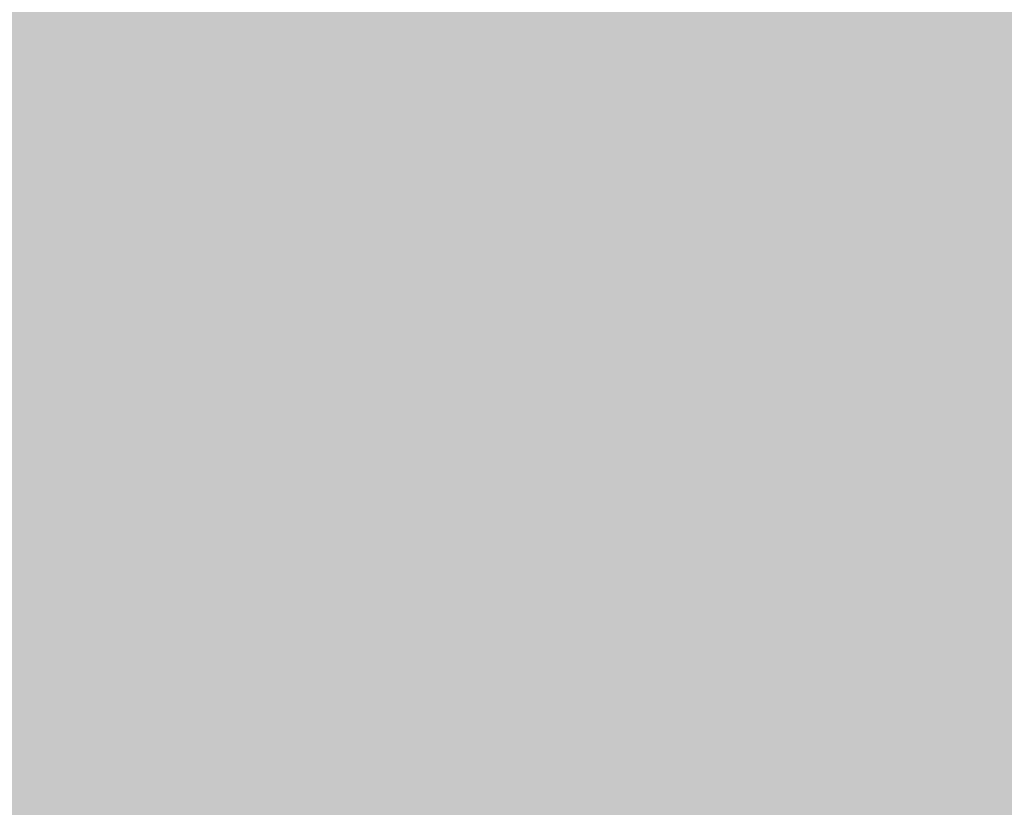
# Model space of a CAD drawing. Units: millimetres. Extents: x -22994 to 29398, y -19990 to 20176.
# Tile 102 of 135: x 229.428 to 231.767, y 85.199 to 87.071. Entities that reach past the tile are written whole.
import ezdxf
from ezdxf import colors
from ezdxf.entities.mleader import LeaderData, LeaderLine
from ezdxf.math import Vec2, Vec3

# ---------------------------------------------------------------- set-up
doc = ezdxf.new("R2010")
doc.units = ezdxf.units.MM
doc.header["$MEASUREMENT"] = 0
doc.layers.add('M-ANNO-TEXT', color=7, linetype='Continuous', lineweight=25)
doc.layers.add('M-DIMS', color=2, linetype='Continuous', lineweight=18)
doc.styles.get("Standard").update_dxf_attribs({"font": 'arial.ttf'})
doc.dimstyles.get("Standard").update_dxf_attribs({"dimtxt": 0.18, "dimasz": 10000, "dimexe": 0.18, "dimexo": 0.0625, "dimgap": 0.09, "dimtad": 0, "dimtih": 1, "dimtoh": 1, "dimdec": 0, "dimzin": 0, "dimdsep": 46, "dimtxsty": 'Standard', "dimcen": 0.09, "dimadec": 0, "dimazin": 0, "dimtfac": 1, "dimtdec": 0, "dimtofl": 0, "dimtmove": 0, "dimatfit": 3, "dimfxl": 1, "dimtolj": 1, "dimtzin": 0, "dimlwd": 30, "dimarcsym": 0})

# ---------------------------------------------------------------- blocks, each defined once
blk = doc.blocks.new('*D2')
at = {"layer": 'Defpoints', "color": 0, "transparency": 16777216}
for p in [(6.6773, 10.2713), (290.852, 10.2713), (290.852, -5.0787)]:
    blk.add_point(p, dxfattribs=at)
at = {"layer": 'M-DIMS', "color": 0, "lineweight": -2, "transparency": 16777216}
for p, q in [((6.6773, 10.2088), (6.6773, -5.2587)), ((290.852, 10.2088), (290.852, -5.2587))]:
    blk.add_line(p, q, dxfattribs=at)
at = {"layer": 'M-DIMS', "color": 0, "lineweight": 30, "transparency": 16777216}
for p, q in [((-9993.3227, -5.0787), (-19993.3227, -5.0787)), ((10290.852, -5.0787), (20290.852, -5.0787))]:
    blk.add_line(p, q, dxfattribs=at)
at = {"layer": 'M-DIMS', "color": 0, "transparency": 16777216}
for points in [[(-9993.3227, 1661.5879), (-9993.3227, -1671.7454), (6.6773, -5.0787)], [(10290.852, 1661.5879), (10290.852, -1671.7454), (290.852, -5.0787)]]:
    blk.add_solid(points, dxfattribs=at)
at = {"layer": 'M-DIMS', "color": 0, "transparency": 16777216, "insert": (148.7647, -5.0787), "char_height": 0.18, "attachment_point": 5}
blk.add_mtext('\\A1;284.2', dxfattribs=at)
blk = doc.blocks.new('*D3')
at = {"layer": 'Defpoints', "color": 0, "transparency": 16777216}
for p in [(110.2647, 204.1654), (110.2647, 176.3662), (95.8327, 127.967)]:
    blk.add_point(p, dxfattribs=at)
at = {"layer": 'M-DIMS', "color": 0, "lineweight": -2, "transparency": 16777216}
for p, q in [((95.8327, 128.0295), (95.8327, 204.3454)), ((110.2647, 176.4287), (110.2647, 204.3454))]:
    blk.add_line(p, q, dxfattribs=at)
at = {"layer": 'M-DIMS', "color": 0, "lineweight": 30, "transparency": 16777216}
for p, q in [((-9904.1673, 204.1654), (-19904.1673, 204.1654)), ((10110.2647, 204.1654), (20110.2647, 204.1654))]:
    blk.add_line(p, q, dxfattribs=at)
at = {"layer": 'M-DIMS', "color": 0, "transparency": 16777216}
for points in [[(-9904.1673, 1870.8321), (-9904.1673, -1462.5013), (95.8327, 204.1654)], [(10110.2647, 1870.8321), (10110.2647, -1462.5013), (110.2647, 204.1654)]]:
    blk.add_solid(points, dxfattribs=at)
at = {"layer": 'M-DIMS', "color": 0, "transparency": 16777216, "insert": (103.0487, 204.1654), "char_height": 0.18, "attachment_point": 5}
blk.add_mtext('\\A1;14.432', dxfattribs=at)
blk = doc.blocks.new('*D4')
at = {"layer": 'Defpoints', "color": 0, "transparency": 16777216}
for p in [(116.2647, 204.1654), (110.2647, 176.3662), (116.2647, 176.3662)]:
    blk.add_point(p, dxfattribs=at)
at = {"layer": 'M-DIMS', "color": 0, "lineweight": -2, "transparency": 16777216}
for p, q in [((110.2647, 176.4287), (110.2647, 204.3454)), ((116.2647, 176.4287), (116.2647, 204.3454))]:
    blk.add_line(p, q, dxfattribs=at)
at = {"layer": 'M-DIMS', "color": 0, "lineweight": 30, "transparency": 16777216}
for p, q in [((-9889.7353, 204.1654), (-19889.7353, 204.1654)), ((10116.2647, 204.1654), (20116.2647, 204.1654))]:
    blk.add_line(p, q, dxfattribs=at)
at = {"layer": 'M-DIMS', "color": 0, "transparency": 16777216}
for points in [[(-9889.7353, 1870.8321), (-9889.7353, -1462.5013), (110.2647, 204.1654)], [(10116.2647, 1870.8321), (10116.2647, -1462.5013), (116.2647, 204.1654)]]:
    blk.add_solid(points, dxfattribs=at)
at = {"layer": 'M-DIMS', "color": 0, "transparency": 16777216, "insert": (113.2647, 204.1654), "char_height": 0.18, "attachment_point": 5}
blk.add_mtext('\\A1;6', dxfattribs=at)
blk = doc.blocks.new('*D5')
at = {"layer": 'Defpoints', "color": 0, "transparency": 16777216}
for p in [(181.2647, 204.1654), (116.2647, 176.3662), (181.2647, 176.3662)]:
    blk.add_point(p, dxfattribs=at)
at = {"layer": 'M-DIMS', "color": 0, "lineweight": -2, "transparency": 16777216}
for p, q in [((116.2647, 176.4287), (116.2647, 204.3454)), ((181.2647, 176.4287), (181.2647, 204.3454))]:
    blk.add_line(p, q, dxfattribs=at)
at = {"layer": 'M-DIMS', "color": 0, "lineweight": 30, "transparency": 16777216}
for p, q in [((-9883.7353, 204.1654), (-19883.7353, 204.1654)), ((10181.2647, 204.1654), (20181.2647, 204.1654))]:
    blk.add_line(p, q, dxfattribs=at)
at = {"layer": 'M-DIMS', "color": 0, "transparency": 16777216}
for points in [[(-9883.7353, 1870.8321), (-9883.7353, -1462.5013), (116.2647, 204.1654)], [(10181.2647, 1870.8321), (10181.2647, -1462.5013), (181.2647, 204.1654)]]:
    blk.add_solid(points, dxfattribs=at)
at = {"layer": 'M-DIMS', "color": 0, "transparency": 16777216, "insert": (148.7647, 204.1654), "char_height": 0.18, "attachment_point": 5}
blk.add_mtext('\\A1;65', dxfattribs=at)
blk = doc.blocks.new('*D6')
at = {"layer": 'Defpoints', "color": 0, "transparency": 16777216}
for p in [(187.2647, 204.1654), (181.2647, 176.3662), (187.2647, 176.3662)]:
    blk.add_point(p, dxfattribs=at)
at = {"layer": 'M-DIMS', "color": 0, "lineweight": -2, "transparency": 16777216}
for p, q in [((181.2647, 176.4287), (181.2647, 204.3454)), ((187.2647, 176.4287), (187.2647, 204.3454))]:
    blk.add_line(p, q, dxfattribs=at)
at = {"layer": 'M-DIMS', "color": 0, "lineweight": 30, "transparency": 16777216}
for p, q in [((-9818.7353, 204.1654), (-19818.7353, 204.1654)), ((10187.2647, 204.1654), (20187.2647, 204.1654))]:
    blk.add_line(p, q, dxfattribs=at)
at = {"layer": 'M-DIMS', "color": 0, "transparency": 16777216}
for points in [[(-9818.7353, 1870.8321), (-9818.7353, -1462.5013), (181.2647, 204.1654)], [(10187.2647, 1870.8321), (10187.2647, -1462.5013), (187.2647, 204.1654)]]:
    blk.add_solid(points, dxfattribs=at)
at = {"layer": 'M-DIMS', "color": 0, "transparency": 16777216, "insert": (184.2647, 204.1654), "char_height": 0.18, "attachment_point": 5}
blk.add_mtext('\\A1;6', dxfattribs=at)
blk = doc.blocks.new('*D7')
at = {"layer": 'Defpoints', "color": 0, "transparency": 16777216}
for p in [(201.6967, 204.1654), (187.2647, 176.3662), (201.6967, 127.967)]:
    blk.add_point(p, dxfattribs=at)
at = {"layer": 'M-DIMS', "color": 0, "lineweight": -2, "transparency": 16777216}
for p, q in [((187.2647, 176.4287), (187.2647, 204.3454)), ((201.6967, 128.0295), (201.6967, 204.3454))]:
    blk.add_line(p, q, dxfattribs=at)
at = {"layer": 'M-DIMS', "color": 0, "lineweight": 30, "transparency": 16777216}
for p, q in [((-9812.7353, 204.1654), (-19812.7353, 204.1654)), ((10201.6967, 204.1654), (20201.6967, 204.1654))]:
    blk.add_line(p, q, dxfattribs=at)
at = {"layer": 'M-DIMS', "color": 0, "transparency": 16777216}
for points in [[(-9812.7353, 1870.8321), (-9812.7353, -1462.5013), (187.2647, 204.1654)], [(10201.6967, 1870.8321), (10201.6967, -1462.5013), (201.6967, 204.1654)]]:
    blk.add_solid(points, dxfattribs=at)
at = {"layer": 'M-DIMS', "color": 0, "transparency": 16777216, "insert": (194.4807, 204.1654), "char_height": 0.18, "attachment_point": 5}
blk.add_mtext('\\A1;14.432', dxfattribs=at)
blk = doc.blocks.new('*D8')
at = {"layer": 'Defpoints', "color": 0, "transparency": 16777216}
for p in [(227.6485, 204.1654), (227.6485, 146.7296), (201.6967, 127.967)]:
    blk.add_point(p, dxfattribs=at)
at = {"layer": 'M-DIMS', "color": 0, "lineweight": -2, "transparency": 16777216}
for p, q in [((201.6967, 128.0295), (201.6967, 204.3454)), ((227.6485, 146.7921), (227.6485, 204.3454))]:
    blk.add_line(p, q, dxfattribs=at)
at = {"layer": 'M-DIMS', "color": 0, "lineweight": 30, "transparency": 16777216}
for p, q in [((-9798.3033, 204.1654), (-19798.3033, 204.1654)), ((10227.6485, 204.1654), (20227.6485, 204.1654))]:
    blk.add_line(p, q, dxfattribs=at)
at = {"layer": 'M-DIMS', "color": 0, "transparency": 16777216}
for points in [[(-9798.3033, 1870.8321), (-9798.3033, -1462.5013), (201.6967, 204.1654)], [(10227.6485, 1870.8321), (10227.6485, -1462.5013), (227.6485, 204.1654)]]:
    blk.add_solid(points, dxfattribs=at)
at = {"layer": 'M-DIMS', "color": 0, "transparency": 16777216, "insert": (214.6726, 204.1654), "char_height": 0.18, "attachment_point": 5}
blk.add_mtext('\\A1;25.95', dxfattribs=at)
blk = doc.blocks.new('*D9')
at = {"layer": 'Defpoints', "color": 0, "transparency": 16777216}
for p in [(187.2647, 176.3662), (306.202, 176.3662), (290.852, 10.2713)]:
    blk.add_point(p, dxfattribs=at)
at = {"layer": 'M-DIMS', "color": 0, "lineweight": 30, "transparency": 16777216}
for p, q in [((306.202, 10176.3662), (306.202, 20176.3662)), ((306.202, -9989.7287), (306.202, -19989.7287))]:
    blk.add_line(p, q, dxfattribs=at)
at = {"layer": 'M-DIMS', "color": 0, "lineweight": -2, "transparency": 16777216}
for p, q in [((187.3272, 176.3662), (306.382, 176.3662)), ((290.9145, 10.2713), (306.382, 10.2713))]:
    blk.add_line(p, q, dxfattribs=at)
at = {"layer": 'M-DIMS', "color": 0, "transparency": 16777216}
for points in [[(-1360.4646, 10176.3662), (1972.8687, 10176.3662), (306.202, 176.3662)], [(-1360.4646, -9989.7287), (1972.8687, -9989.7287), (306.202, 10.2713)]]:
    blk.add_solid(points, dxfattribs=at)
at = {"layer": 'M-DIMS', "color": 0, "transparency": 16777216, "insert": (306.202, 93.3187), "char_height": 0.18, "attachment_point": 5}
blk.add_mtext('\\A1;166.1', dxfattribs=at)
blk = doc.blocks.new('*D10')
at = {"layer": 'Defpoints', "color": 0, "transparency": 16777216}
for p in [(125.6498, 136.0713), (133.3459, 136.0713), (133.3459, -5.0787)]:
    blk.add_point(p, dxfattribs=at)
at = {"layer": 'M-DIMS', "color": 0, "lineweight": -2, "transparency": 16777216}
for p, q in [((125.6498, 136.0088), (125.6498, -5.2587)), ((133.3459, 136.0088), (133.3459, -5.2587))]:
    blk.add_line(p, q, dxfattribs=at)
at = {"layer": 'M-DIMS', "color": 0, "lineweight": 30, "transparency": 16777216}
for p, q in [((-9874.3502, -5.0787), (-19874.3502, -5.0787)), ((10133.3459, -5.0787), (20133.3459, -5.0787))]:
    blk.add_line(p, q, dxfattribs=at)
at = {"layer": 'M-DIMS', "color": 0, "transparency": 16777216}
for points in [[(-9874.3502, 1661.5879), (-9874.3502, -1671.7454), (125.6498, -5.0787)], [(10133.3459, 1661.5879), (10133.3459, -1671.7454), (133.3459, -5.0787)]]:
    blk.add_solid(points, dxfattribs=at)
at = {"layer": 'M-DIMS', "color": 0, "transparency": 16777216, "insert": (129.4978, -5.0787), "char_height": 0.18, "attachment_point": 5}
blk.add_mtext('\\A1;7.696', dxfattribs=at)
blk = doc.blocks.new('*D11')
at = {"layer": 'Defpoints', "color": 0, "transparency": 16777216}
for p in [(133.3459, 136.0713), (135.6498, 136.0713), (135.6498, -5.0787)]:
    blk.add_point(p, dxfattribs=at)
at = {"layer": 'M-DIMS', "color": 0, "lineweight": -2, "transparency": 16777216}
for p, q in [((133.3459, 136.0088), (133.3459, -5.2587)), ((135.6498, 136.0088), (135.6498, -5.2587))]:
    blk.add_line(p, q, dxfattribs=at)
at = {"layer": 'M-DIMS', "color": 0, "lineweight": 30, "transparency": 16777216}
for p, q in [((-9866.6541, -5.0787), (-19866.6541, -5.0787)), ((10135.6498, -5.0787), (20135.6498, -5.0787))]:
    blk.add_line(p, q, dxfattribs=at)
at = {"layer": 'M-DIMS', "color": 0, "transparency": 16777216}
for points in [[(-9866.6541, 1661.5879), (-9866.6541, -1671.7454), (133.3459, -5.0787)], [(10135.6498, 1661.5879), (10135.6498, -1671.7454), (135.6498, -5.0787)]]:
    blk.add_solid(points, dxfattribs=at)
at = {"layer": 'M-DIMS', "color": 0, "transparency": 16777216, "insert": (134.4978, -5.0787), "char_height": 0.18, "attachment_point": 5}
blk.add_mtext('\\A1;2.304', dxfattribs=at)
blk = doc.blocks.new('*D12')
at = {"layer": 'Defpoints', "color": 0, "transparency": 16777216}
for p in [(135.6498, 136.0713), (145.6498, 136.0713), (145.6498, -5.0787)]:
    blk.add_point(p, dxfattribs=at)
at = {"layer": 'M-DIMS', "color": 0, "lineweight": -2, "transparency": 16777216}
for p, q in [((135.6498, 136.0088), (135.6498, -5.2587)), ((145.6498, 136.0088), (145.6498, -5.2587))]:
    blk.add_line(p, q, dxfattribs=at)
at = {"layer": 'M-DIMS', "color": 0, "lineweight": 30, "transparency": 16777216}
for p, q in [((-9864.3502, -5.0787), (-19864.3502, -5.0787)), ((10145.6498, -5.0787), (20145.6498, -5.0787))]:
    blk.add_line(p, q, dxfattribs=at)
at = {"layer": 'M-DIMS', "color": 0, "transparency": 16777216}
for points in [[(-9864.3502, 1661.5879), (-9864.3502, -1671.7454), (135.6498, -5.0787)], [(10145.6498, 1661.5879), (10145.6498, -1671.7454), (145.6498, -5.0787)]]:
    blk.add_solid(points, dxfattribs=at)
at = {"layer": 'M-DIMS', "color": 0, "transparency": 16777216, "insert": (140.6498, -5.0787), "char_height": 0.18, "attachment_point": 5}
blk.add_mtext('\\A1;10', dxfattribs=at)
blk = doc.blocks.new('*D13')
at = {"layer": 'Defpoints', "color": 0, "transparency": 16777216}
for p in [(145.6498, 136.0713), (155.6498, 136.0713), (155.6498, -5.0787)]:
    blk.add_point(p, dxfattribs=at)
at = {"layer": 'M-DIMS', "color": 0, "lineweight": -2, "transparency": 16777216}
for p, q in [((145.6498, 136.0088), (145.6498, -5.2587)), ((155.6498, 136.0088), (155.6498, -5.2587))]:
    blk.add_line(p, q, dxfattribs=at)
at = {"layer": 'M-DIMS', "color": 0, "lineweight": 30, "transparency": 16777216}
for p, q in [((-9854.3502, -5.0787), (-19854.3502, -5.0787)), ((10155.6498, -5.0787), (20155.6498, -5.0787))]:
    blk.add_line(p, q, dxfattribs=at)
at = {"layer": 'M-DIMS', "color": 0, "transparency": 16777216}
for points in [[(-9854.3502, 1661.5879), (-9854.3502, -1671.7454), (145.6498, -5.0787)], [(10155.6498, 1661.5879), (10155.6498, -1671.7454), (155.6498, -5.0787)]]:
    blk.add_solid(points, dxfattribs=at)
at = {"layer": 'M-DIMS', "color": 0, "transparency": 16777216, "insert": (150.6498, -5.0787), "char_height": 0.18, "attachment_point": 5}
blk.add_mtext('\\A1;10', dxfattribs=at)
blk = doc.blocks.new('*D14')
at = {"layer": 'Defpoints', "color": 0, "transparency": 16777216}
for p in [(155.6498, 136.0713), (165.6498, 136.0713), (165.6498, -5.0787)]:
    blk.add_point(p, dxfattribs=at)
at = {"layer": 'M-DIMS', "color": 0, "lineweight": -2, "transparency": 16777216}
for p, q in [((155.6498, 136.0088), (155.6498, -5.2587)), ((165.6498, 136.0088), (165.6498, -5.2587))]:
    blk.add_line(p, q, dxfattribs=at)
at = {"layer": 'M-DIMS', "color": 0, "lineweight": 30, "transparency": 16777216}
for p, q in [((-9844.3502, -5.0787), (-19844.3502, -5.0787)), ((10165.6498, -5.0787), (20165.6498, -5.0787))]:
    blk.add_line(p, q, dxfattribs=at)
at = {"layer": 'M-DIMS', "color": 0, "transparency": 16777216}
for points in [[(-9844.3502, 1661.5879), (-9844.3502, -1671.7454), (155.6498, -5.0787)], [(10165.6498, 1661.5879), (10165.6498, -1671.7454), (165.6498, -5.0787)]]:
    blk.add_solid(points, dxfattribs=at)
at = {"layer": 'M-DIMS', "color": 0, "transparency": 16777216, "insert": (160.6498, -5.0787), "char_height": 0.18, "attachment_point": 5}
blk.add_mtext('\\A1;10', dxfattribs=at)
blk = doc.blocks.new('*D15')
at = {"layer": 'Defpoints', "color": 0, "transparency": 16777216}
for p in [(173.3459, 154.788), (173.3459, 136.0713), (306.202, 136.0713)]:
    blk.add_point(p, dxfattribs=at)
at = {"layer": 'M-DIMS', "color": 0, "lineweight": 30, "transparency": 16777216}
for p, q in [((306.202, 10154.788), (306.202, 20154.788)), ((306.202, -9863.9287), (306.202, -19863.9287))]:
    blk.add_line(p, q, dxfattribs=at)
at = {"layer": 'M-DIMS', "color": 0, "lineweight": -2, "transparency": 16777216}
for p, q in [((173.4084, 154.788), (306.382, 154.788)), ((173.4084, 136.0713), (306.382, 136.0713))]:
    blk.add_line(p, q, dxfattribs=at)
at = {"layer": 'M-DIMS', "color": 0, "transparency": 16777216}
for points in [[(-1360.4646, 10154.788), (1972.8687, 10154.788), (306.202, 154.788)], [(-1360.4646, -9863.9287), (1972.8687, -9863.9287), (306.202, 136.0713)]]:
    blk.add_solid(points, dxfattribs=at)
at = {"layer": 'M-DIMS', "color": 0, "transparency": 16777216, "insert": (306.202, 145.4297), "char_height": 0.18, "attachment_point": 5}
blk.add_mtext('\\A1;18.717', dxfattribs=at)
blk = doc.blocks.new('*D16')
at = {"layer": 'Defpoints', "color": 0, "transparency": 16777216}
for p in [(120.1702, 204.1654), (110.4658, 48.0349), (120.1702, 48.0349)]:
    blk.add_point(p, dxfattribs=at)
at = {"layer": 'M-DIMS', "color": 0, "lineweight": -2, "transparency": 16777216}
for p, q in [((110.4658, 48.0974), (110.4658, 204.3454)), ((120.1702, 48.0974), (120.1702, 204.3454))]:
    blk.add_line(p, q, dxfattribs=at)
at = {"layer": 'M-DIMS', "color": 0, "lineweight": 30, "transparency": 16777216}
for p, q in [((-9889.5342, 204.1654), (-19889.5342, 204.1654)), ((10120.1702, 204.1654), (20120.1702, 204.1654))]:
    blk.add_line(p, q, dxfattribs=at)
at = {"layer": 'M-DIMS', "color": 0, "transparency": 16777216}
for points in [[(-9889.5342, 1870.8321), (-9889.5342, -1462.5013), (110.4658, 204.1654)], [(10120.1702, 1870.8321), (10120.1702, -1462.5013), (120.1702, 204.1654)]]:
    blk.add_solid(points, dxfattribs=at)
at = {"layer": 'M-DIMS', "color": 0, "transparency": 16777216, "insert": (115.318, 204.1654), "char_height": 0.18, "attachment_point": 5}
blk.add_mtext('\\A1;9.704', dxfattribs=at)
blk = doc.blocks.new('*D17')
at = {"layer": 'Defpoints', "color": 0, "transparency": 16777216}
for p in [(126.1702, 204.1654), (120.1702, 48.0349), (126.1702, 48.0349)]:
    blk.add_point(p, dxfattribs=at)
at = {"layer": 'M-DIMS', "color": 0, "lineweight": -2, "transparency": 16777216}
for p, q in [((120.1702, 48.0974), (120.1702, 204.3454)), ((126.1702, 48.0974), (126.1702, 204.3454))]:
    blk.add_line(p, q, dxfattribs=at)
at = {"layer": 'M-DIMS', "color": 0, "lineweight": 30, "transparency": 16777216}
for p, q in [((-9879.8298, 204.1654), (-19879.8298, 204.1654)), ((10126.1702, 204.1654), (20126.1702, 204.1654))]:
    blk.add_line(p, q, dxfattribs=at)
at = {"layer": 'M-DIMS', "color": 0, "transparency": 16777216}
for points in [[(-9879.8298, 1870.8321), (-9879.8298, -1462.5013), (120.1702, 204.1654)], [(10126.1702, 1870.8321), (10126.1702, -1462.5013), (126.1702, 204.1654)]]:
    blk.add_solid(points, dxfattribs=at)
at = {"layer": 'M-DIMS', "color": 0, "transparency": 16777216, "insert": (123.1702, 204.1654), "char_height": 0.18, "attachment_point": 5}
blk.add_mtext('\\A1;6', dxfattribs=at)
blk = doc.blocks.new('*D18')
at = {"layer": 'Defpoints', "color": 0, "transparency": 16777216}
for p in [(132.1702, 204.1654), (126.1702, 48.0349), (132.1702, 48.0349)]:
    blk.add_point(p, dxfattribs=at)
at = {"layer": 'M-DIMS', "color": 0, "lineweight": -2, "transparency": 16777216}
for p, q in [((126.1702, 48.0974), (126.1702, 204.3454)), ((132.1702, 48.0974), (132.1702, 204.3454))]:
    blk.add_line(p, q, dxfattribs=at)
at = {"layer": 'M-DIMS', "color": 0, "lineweight": 30, "transparency": 16777216}
for p, q in [((-9873.8298, 204.1654), (-19873.8298, 204.1654)), ((10132.1702, 204.1654), (20132.1702, 204.1654))]:
    blk.add_line(p, q, dxfattribs=at)
at = {"layer": 'M-DIMS', "color": 0, "transparency": 16777216}
for points in [[(-9873.8298, 1870.8321), (-9873.8298, -1462.5013), (126.1702, 204.1654)], [(10132.1702, 1870.8321), (10132.1702, -1462.5013), (132.1702, 204.1654)]]:
    blk.add_solid(points, dxfattribs=at)
at = {"layer": 'M-DIMS', "color": 0, "transparency": 16777216, "insert": (129.1702, 204.1654), "char_height": 0.18, "attachment_point": 5}
blk.add_mtext('\\A1;6', dxfattribs=at)
blk = doc.blocks.new('*D19')
at = {"layer": 'Defpoints', "color": 0, "transparency": 16777216}
for p in [(138.1702, 204.1654), (132.1702, 48.0349), (138.1702, 48.0349)]:
    blk.add_point(p, dxfattribs=at)
at = {"layer": 'M-DIMS', "color": 0, "lineweight": -2, "transparency": 16777216}
for p, q in [((132.1702, 48.0974), (132.1702, 204.3454)), ((138.1702, 48.0974), (138.1702, 204.3454))]:
    blk.add_line(p, q, dxfattribs=at)
at = {"layer": 'M-DIMS', "color": 0, "lineweight": 30, "transparency": 16777216}
for p, q in [((-9867.8298, 204.1654), (-19867.8298, 204.1654)), ((10138.1702, 204.1654), (20138.1702, 204.1654))]:
    blk.add_line(p, q, dxfattribs=at)
at = {"layer": 'M-DIMS', "color": 0, "transparency": 16777216}
for points in [[(-9867.8298, 1870.8321), (-9867.8298, -1462.5013), (132.1702, 204.1654)], [(10138.1702, 1870.8321), (10138.1702, -1462.5013), (138.1702, 204.1654)]]:
    blk.add_solid(points, dxfattribs=at)
at = {"layer": 'M-DIMS', "color": 0, "transparency": 16777216, "insert": (135.1702, 204.1654), "char_height": 0.18, "attachment_point": 5}
blk.add_mtext('\\A1;6', dxfattribs=at)
blk = doc.blocks.new('*D20')
at = {"layer": 'Defpoints', "color": 0, "transparency": 16777216}
for p in [(144.1702, 204.1654), (138.1702, 48.0349), (144.1702, 48.0349)]:
    blk.add_point(p, dxfattribs=at)
at = {"layer": 'M-DIMS', "color": 0, "lineweight": -2, "transparency": 16777216}
for p, q in [((138.1702, 48.0974), (138.1702, 204.3454)), ((144.1702, 48.0974), (144.1702, 204.3454))]:
    blk.add_line(p, q, dxfattribs=at)
at = {"layer": 'M-DIMS', "color": 0, "lineweight": 30, "transparency": 16777216}
for p, q in [((-9861.8298, 204.1654), (-19861.8298, 204.1654)), ((10144.1702, 204.1654), (20144.1702, 204.1654))]:
    blk.add_line(p, q, dxfattribs=at)
at = {"layer": 'M-DIMS', "color": 0, "transparency": 16777216}
for points in [[(-9861.8298, 1870.8321), (-9861.8298, -1462.5013), (138.1702, 204.1654)], [(10144.1702, 1870.8321), (10144.1702, -1462.5013), (144.1702, 204.1654)]]:
    blk.add_solid(points, dxfattribs=at)
at = {"layer": 'M-DIMS', "color": 0, "transparency": 16777216, "insert": (141.1702, 204.1654), "char_height": 0.18, "attachment_point": 5}
blk.add_mtext('\\A1;6', dxfattribs=at)
blk = doc.blocks.new('*D21')
at = {"layer": 'Defpoints', "color": 0, "transparency": 16777216}
for p in [(149.1157, 204.1654), (144.1702, 48.0349), (149.1157, 48.0349)]:
    blk.add_point(p, dxfattribs=at)
at = {"layer": 'M-DIMS', "color": 0, "lineweight": -2, "transparency": 16777216}
for p, q in [((144.1702, 48.0974), (144.1702, 204.3454)), ((149.1157, 48.0974), (149.1157, 204.3454))]:
    blk.add_line(p, q, dxfattribs=at)
at = {"layer": 'M-DIMS', "color": 0, "lineweight": 30, "transparency": 16777216}
for p, q in [((-9855.8298, 204.1654), (-19855.8298, 204.1654)), ((10149.1157, 204.1654), (20149.1157, 204.1654))]:
    blk.add_line(p, q, dxfattribs=at)
at = {"layer": 'M-DIMS', "color": 0, "transparency": 16777216}
for points in [[(-9855.8298, 1870.8321), (-9855.8298, -1462.5013), (144.1702, 204.1654)], [(10149.1157, 1870.8321), (10149.1157, -1462.5013), (149.1157, 204.1654)]]:
    blk.add_solid(points, dxfattribs=at)
at = {"layer": 'M-DIMS', "color": 0, "transparency": 16777216, "insert": (146.6429, 204.1654), "char_height": 0.18, "attachment_point": 5}
blk.add_mtext('\\A1;4.945', dxfattribs=at)
blk = doc.blocks.new('*D22')
at = {"layer": 'Defpoints', "color": 0, "transparency": 16777216}
for p in [(149.1157, 30.9895), (155.1157, 30.9895), (155.1157, -5.0787)]:
    blk.add_point(p, dxfattribs=at)
at = {"layer": 'M-DIMS', "color": 0, "lineweight": -2, "transparency": 16777216}
for p, q in [((149.1157, 30.927), (149.1157, -5.2587)), ((155.1157, 30.927), (155.1157, -5.2587))]:
    blk.add_line(p, q, dxfattribs=at)
at = {"layer": 'M-DIMS', "color": 0, "lineweight": 30, "transparency": 16777216}
for p, q in [((-9850.8843, -5.0787), (-19850.8843, -5.0787)), ((10155.1157, -5.0787), (20155.1157, -5.0787))]:
    blk.add_line(p, q, dxfattribs=at)
at = {"layer": 'M-DIMS', "color": 0, "transparency": 16777216}
for points in [[(-9850.8843, 1661.5879), (-9850.8843, -1671.7454), (149.1157, -5.0787)], [(10155.1157, 1661.5879), (10155.1157, -1671.7454), (155.1157, -5.0787)]]:
    blk.add_solid(points, dxfattribs=at)
at = {"layer": 'M-DIMS', "color": 0, "transparency": 16777216, "insert": (152.1157, -5.0787), "char_height": 0.18, "attachment_point": 5}
blk.add_mtext('\\A1;6', dxfattribs=at)
blk = doc.blocks.new('*D23')
at = {"layer": 'Defpoints', "color": 0, "transparency": 16777216}
for p in [(155.1157, 30.9895), (161.1157, 30.9895), (161.1157, -5.0787)]:
    blk.add_point(p, dxfattribs=at)
at = {"layer": 'M-DIMS', "color": 0, "lineweight": -2, "transparency": 16777216}
for p, q in [((155.1157, 30.927), (155.1157, -5.2587)), ((161.1157, 30.927), (161.1157, -5.2587))]:
    blk.add_line(p, q, dxfattribs=at)
at = {"layer": 'M-DIMS', "color": 0, "lineweight": 30, "transparency": 16777216}
for p, q in [((-9844.8843, -5.0787), (-19844.8843, -5.0787)), ((10161.1157, -5.0787), (20161.1157, -5.0787))]:
    blk.add_line(p, q, dxfattribs=at)
at = {"layer": 'M-DIMS', "color": 0, "transparency": 16777216}
for points in [[(-9844.8843, 1661.5879), (-9844.8843, -1671.7454), (155.1157, -5.0787)], [(10161.1157, 1661.5879), (10161.1157, -1671.7454), (161.1157, -5.0787)]]:
    blk.add_solid(points, dxfattribs=at)
at = {"layer": 'M-DIMS', "color": 0, "transparency": 16777216, "insert": (158.1157, -5.0787), "char_height": 0.18, "attachment_point": 5}
blk.add_mtext('\\A1;6', dxfattribs=at)
blk = doc.blocks.new('*D24')
at = {"layer": 'Defpoints', "color": 0, "transparency": 16777216}
for p in [(161.1157, 30.9895), (166.4387, 30.9895), (166.4387, -5.0787)]:
    blk.add_point(p, dxfattribs=at)
at = {"layer": 'M-DIMS', "color": 0, "lineweight": -2, "transparency": 16777216}
for p, q in [((161.1157, 30.927), (161.1157, -5.2587)), ((166.4387, 30.927), (166.4387, -5.2587))]:
    blk.add_line(p, q, dxfattribs=at)
at = {"layer": 'M-DIMS', "color": 0, "lineweight": 30, "transparency": 16777216}
for p, q in [((-9838.8843, -5.0787), (-19838.8843, -5.0787)), ((10166.4387, -5.0787), (20166.4387, -5.0787))]:
    blk.add_line(p, q, dxfattribs=at)
at = {"layer": 'M-DIMS', "color": 0, "transparency": 16777216}
for points in [[(-9838.8843, 1661.5879), (-9838.8843, -1671.7454), (161.1157, -5.0787)], [(10166.4387, 1661.5879), (10166.4387, -1671.7454), (166.4387, -5.0787)]]:
    blk.add_solid(points, dxfattribs=at)
at = {"layer": 'M-DIMS', "color": 0, "transparency": 16777216, "insert": (163.7772, -5.0787), "char_height": 0.18, "attachment_point": 5}
blk.add_mtext('\\A1;5.323', dxfattribs=at)
blk = doc.blocks.new('*D25')
at = {"layer": 'Defpoints', "color": 0, "transparency": 16777216}
for p in [(166.4387, 30.9895), (172.4387, 30.9895), (172.4387, -5.0787)]:
    blk.add_point(p, dxfattribs=at)
at = {"layer": 'M-DIMS', "color": 0, "lineweight": -2, "transparency": 16777216}
for p, q in [((166.4387, 30.927), (166.4387, -5.2587)), ((172.4387, 30.927), (172.4387, -5.2587))]:
    blk.add_line(p, q, dxfattribs=at)
at = {"layer": 'M-DIMS', "color": 0, "lineweight": 30, "transparency": 16777216}
for p, q in [((-9833.5613, -5.0787), (-19833.5613, -5.0787)), ((10172.4387, -5.0787), (20172.4387, -5.0787))]:
    blk.add_line(p, q, dxfattribs=at)
at = {"layer": 'M-DIMS', "color": 0, "transparency": 16777216}
for points in [[(-9833.5613, 1661.5879), (-9833.5613, -1671.7454), (166.4387, -5.0787)], [(10172.4387, 1661.5879), (10172.4387, -1671.7454), (172.4387, -5.0787)]]:
    blk.add_solid(points, dxfattribs=at)
at = {"layer": 'M-DIMS', "color": 0, "transparency": 16777216, "insert": (169.4387, -5.0787), "char_height": 0.18, "attachment_point": 5}
blk.add_mtext('\\A1;6', dxfattribs=at)
blk = doc.blocks.new('*D26')
at = {"layer": 'Defpoints', "color": 0, "transparency": 16777216}
for p in [(172.4387, 30.9895), (178.4387, 30.9895), (178.4387, -5.0787)]:
    blk.add_point(p, dxfattribs=at)
at = {"layer": 'M-DIMS', "color": 0, "lineweight": -2, "transparency": 16777216}
for p, q in [((172.4387, 30.927), (172.4387, -5.2587)), ((178.4387, 30.927), (178.4387, -5.2587))]:
    blk.add_line(p, q, dxfattribs=at)
at = {"layer": 'M-DIMS', "color": 0, "lineweight": 30, "transparency": 16777216}
for p, q in [((-9827.5613, -5.0787), (-19827.5613, -5.0787)), ((10178.4387, -5.0787), (20178.4387, -5.0787))]:
    blk.add_line(p, q, dxfattribs=at)
at = {"layer": 'M-DIMS', "color": 0, "transparency": 16777216}
for points in [[(-9827.5613, 1661.5879), (-9827.5613, -1671.7454), (172.4387, -5.0787)], [(10178.4387, 1661.5879), (10178.4387, -1671.7454), (178.4387, -5.0787)]]:
    blk.add_solid(points, dxfattribs=at)
at = {"layer": 'M-DIMS', "color": 0, "transparency": 16777216, "insert": (175.4387, -5.0787), "char_height": 0.18, "attachment_point": 5}
blk.add_mtext('\\A1;6', dxfattribs=at)
blk = doc.blocks.new('*D27')
at = {"layer": 'Defpoints', "color": 0, "transparency": 16777216}
for p in [(178.4387, 30.9895), (188.1175, 30.9895), (188.1175, -5.0787)]:
    blk.add_point(p, dxfattribs=at)
at = {"layer": 'M-DIMS', "color": 0, "lineweight": -2, "transparency": 16777216}
for p, q in [((178.4387, 30.927), (178.4387, -5.2587)), ((188.1175, 30.927), (188.1175, -5.2587))]:
    blk.add_line(p, q, dxfattribs=at)
at = {"layer": 'M-DIMS', "color": 0, "lineweight": 30, "transparency": 16777216}
for p, q in [((-9821.5613, -5.0787), (-19821.5613, -5.0787)), ((10188.1175, -5.0787), (20188.1175, -5.0787))]:
    blk.add_line(p, q, dxfattribs=at)
at = {"layer": 'M-DIMS', "color": 0, "transparency": 16777216}
for points in [[(-9821.5613, 1661.5879), (-9821.5613, -1671.7454), (178.4387, -5.0787)], [(10188.1175, 1661.5879), (10188.1175, -1671.7454), (188.1175, -5.0787)]]:
    blk.add_solid(points, dxfattribs=at)
at = {"layer": 'M-DIMS', "color": 0, "transparency": 16777216, "insert": (183.2781, -5.0787), "char_height": 0.18, "attachment_point": 5}
blk.add_mtext('\\A1;9.679', dxfattribs=at)
blk = doc.blocks.new('*D28')
at = {"layer": 'Defpoints', "color": 0, "transparency": 16777216}
for p in [(188.1175, 48.0349), (306.202, 48.0349), (188.1175, 30.9895)]:
    blk.add_point(p, dxfattribs=at)
at = {"layer": 'M-DIMS', "color": 0, "lineweight": 30, "transparency": 16777216}
for p, q in [((306.202, 10048.0349), (306.202, 20048.0349)), ((306.202, -9969.0105), (306.202, -19969.0105))]:
    blk.add_line(p, q, dxfattribs=at)
at = {"layer": 'M-DIMS', "color": 0, "lineweight": -2, "transparency": 16777216}
for p, q in [((188.18, 48.0349), (306.382, 48.0349)), ((188.18, 30.9895), (306.382, 30.9895))]:
    blk.add_line(p, q, dxfattribs=at)
at = {"layer": 'M-DIMS', "color": 0, "transparency": 16777216}
for points in [[(-1360.4646, 10048.0349), (1972.8687, 10048.0349), (306.202, 48.0349)], [(-1360.4646, -9969.0105), (1972.8687, -9969.0105), (306.202, 30.9895)]]:
    blk.add_solid(points, dxfattribs=at)
at = {"layer": 'M-DIMS', "color": 0, "transparency": 16777216, "insert": (306.202, 39.5122), "char_height": 0.18, "attachment_point": 5}
blk.add_mtext('\\A1;17.045', dxfattribs=at)
blk = doc.blocks.new('*D29')
at = {"layer": 'Defpoints', "color": 0, "transparency": 16777216}
for p in [(36.8006, 80.045), (64.0296, 80.045)]:
    blk.add_point(p, dxfattribs=at)
at = {"layer": 'M-DIMS', "color": 0, "lineweight": -2, "transparency": 16777216}
for p, q in [((50.4151, 79.955), (50.4151, 80.135)), ((50.3251, 80.045), (50.5051, 80.045))]:
    blk.add_line(p, q, dxfattribs=at)
at = {"layer": 'M-DIMS', "color": 0, "lineweight": 30, "transparency": 16777216}
blk.add_line((20064.0296, 80.0303), (10064.0296, 80.0377), dxfattribs=at)
at = {"layer": 'M-DIMS', "color": 0, "transparency": 16777216}
blk.add_solid([(10064.0309, 1746.7043), (10064.0284, -1586.629), (64.0296, 80.045)], dxfattribs=at)
at = {"layer": 'M-DIMS', "color": 0, "transparency": 16777216, "insert": (20064.5213, 80.0303), "char_height": 0.18, "attachment_point": 5}
blk.add_mtext('\\A1;∅27.23', dxfattribs=at)
blk = doc.blocks.new('*D30')
at = {"layer": 'Defpoints', "color": 0, "transparency": 16777216}
for p in [(216.3148, 146.7291), (238.9821, 146.73)]:
    blk.add_point(p, dxfattribs=at)
at = {"layer": 'M-DIMS', "color": 0, "lineweight": 30, "transparency": 16777216}
blk.add_line((20238.9821, 147.4959), (10238.9821, 147.1129), dxfattribs=at)
at = {"layer": 'M-DIMS', "color": 0, "lineweight": -2, "transparency": 16777216}
for p, q in [((227.6485, 146.6396), (227.6485, 146.8196)), ((227.5585, 146.7296), (227.7385, 146.7296))]:
    blk.add_line(p, q, dxfattribs=at)
at = {"layer": 'M-DIMS', "color": 0, "transparency": 16777216}
blk.add_solid([(10238.9183, 1813.7796), (10239.0459, -1519.5537), (238.9821, 146.73)], dxfattribs=at)
at = {"layer": 'M-DIMS', "color": 0, "transparency": 16777216, "insert": (20239.5436, 147.4959), "char_height": 0.18, "attachment_point": 5}
blk.add_mtext('\\A1;∅22.667', dxfattribs=at)
blk = doc.blocks.new('*D31')
at = {"layer": 'Defpoints', "color": 0, "transparency": 16777216}
for p in [(223.1641, 146.7291), (232.1328, 146.73)]:
    blk.add_point(p, dxfattribs=at)
at = {"layer": 'M-DIMS', "color": 0, "lineweight": 30, "transparency": 16777216}
blk.add_line((20232.1327, 148.6656), (10232.1328, 147.6978), dxfattribs=at)
at = {"layer": 'M-DIMS', "color": 0, "lineweight": -2, "transparency": 16777216}
for p, q in [((227.6485, 146.6396), (227.6485, 146.8196)), ((227.5585, 146.7296), (227.7385, 146.7296))]:
    blk.add_line(p, q, dxfattribs=at)
at = {"layer": 'M-DIMS', "color": 0, "transparency": 16777216}
blk.add_solid([(10231.9715, 1814.3645), (10232.2941, -1518.9688), (232.1328, 146.73)], dxfattribs=at)
at = {"layer": 'M-DIMS', "color": 0, "transparency": 16777216, "insert": (20232.6245, 148.6656), "char_height": 0.18, "attachment_point": 5}
blk.add_mtext('\\A1;∅8.969', dxfattribs=at)
blk = doc.blocks.new('*D33')
at = {"layer": 'Defpoints', "color": 0, "transparency": 16777216}
for p in [(229.5613, 154.3773), (232.9972, 153.3509)]:
    blk.add_point(p, dxfattribs=at)
at = {"layer": 'M-DIMS', "color": 0, "lineweight": -2, "transparency": 16777216}
for p, q in [((229.5613, 154.2873), (229.5613, 154.4673)), ((229.4713, 154.3773), (229.6513, 154.3773))]:
    blk.add_line(p, q, dxfattribs=at)
at = {"layer": 'M-DIMS', "color": 0, "lineweight": 30, "transparency": 16777216}
for p, q in [((19396.3388, -5570.8378), (9814.668, -2708.7434)), ((29396.3388, -5570.8378), (19396.3388, -5570.8378))]:
    blk.add_line(p, q, dxfattribs=at)
at = {"layer": 'M-DIMS', "color": 0, "transparency": 16777216}
blk.add_solid([(10291.6837, -1111.7983), (9337.6523, -4305.6886), (232.9972, 153.3509)], dxfattribs=at)
at = {"layer": 'M-DIMS', "color": 0, "transparency": 16777216, "insert": (29397.0125, -5570.8378), "char_height": 0.18, "attachment_point": 5}
blk.add_mtext('\\A1;6X R3.586', dxfattribs=at)
blk = doc.blocks.new('*D36')
at = {"layer": 'Defpoints', "color": 0, "transparency": 16777216}
for p in [(46.39, 31.3035), (46.3875, 26.5934)]:
    blk.add_point(p, dxfattribs=at)
at = {"layer": 'M-DIMS', "color": 0, "lineweight": 30, "transparency": 16777216}
for p, q in [((57.1499, 20031.3006), (51.77, 10031.302)), ((10057.1499, 20031.3006), (57.1499, 20031.3006))]:
    blk.add_line(p, q, dxfattribs=at)
at = {"layer": 'M-DIMS', "color": 0, "lineweight": -2, "transparency": 16777216}
for p, q in [((46.3887, 28.8585), (46.3887, 29.0385)), ((46.2987, 28.9485), (46.4787, 28.9485))]:
    blk.add_line(p, q, dxfattribs=at)
at = {"layer": 'M-DIMS', "color": 0, "transparency": 16777216}
blk.add_solid([(-1614.8965, 10032.1987), (1718.4364, 10030.4054), (46.39, 31.3035)], dxfattribs=at)
at = {"layer": 'M-DIMS', "color": 0, "transparency": 16777216, "insert": (10057.5542, 20031.3006), "char_height": 0.18, "attachment_point": 5}
blk.add_mtext('\\A1;∅4.71', dxfattribs=at)

msp = doc.modelspace()

# ---------------------------------------------------------------- dimensions: what is measured, and where the dimension line sits
at = {"layer": 'M-DIMS'}
for base, p1, p2, override, picture, middle in [((306.202, 176.3662), (290.852, 10.2713), (187.2647, 176.3662), {"dimdec": 1, "dimlfac": 1, "dimrnd": 0, "dimzin": 0, "dimdsep": 46, "dimlunit": 2}, '*D9', (306.202, 93.3187)), ((306.202, 136.0713), (173.3459, 154.788), (173.3459, 136.0713), {"dimdec": 3, "dimlfac": 1, "dimrnd": 0, "dimzin": 0, "dimdsep": 46, "dimlunit": 2}, '*D15', (306.202, 145.4297)), ((306.202, 48.0349), (188.1175, 30.9895), (188.1175, 48.0349), {"dimdec": 3, "dimlfac": 1, "dimrnd": 0, "dimzin": 0, "dimdsep": 46, "dimlunit": 2}, '*D28', (306.202, 39.5122))]:
    dim = msp.add_linear_dim(base=base, p1=p1, p2=p2, angle=90, dimstyle='Standard', override=override, dxfattribs=at)
    dim.commit()
    dim.dimension.update_dxf_attribs({"geometry": picture, "text_midpoint": middle})
for p1, p2, override, picture, middle in [((46.3875, 26.5934), (46.39, 31.3035), {"dimdec": 2, "dimlfac": 1, "dimrnd": 0, "dimzin": 0, "dimdsep": 46, "dimlunit": 2}, '*D36', (10057.5542, 20031.3006)), ((223.1641, 146.7291), (232.1328, 146.73), {"dimdec": 3, "dimlfac": 1, "dimrnd": 0, "dimzin": 0, "dimdsep": 46, "dimlunit": 2}, '*D31', (20232.1327, 148.6656)), ((216.3148, 146.7291), (238.9821, 146.73), {"dimdec": 3, "dimlfac": 1, "dimrnd": 0, "dimzin": 0, "dimdsep": 46, "dimlunit": 2}, '*D30', (20238.9821, 147.4959))]:
    dim = msp.add_diameter_dim_2p(p1=p1, p2=p2, dimstyle='Standard', override=override, dxfattribs=at)
    dim.commit()
    dim.dimension.update_dxf_attribs({"geometry": picture, "text_midpoint": middle, "dimtype": 163})
for base, p1, p2, override, picture, middle in [((110.2647, 204.1654), (95.8327, 127.967), (110.2647, 176.3662), {"dimdec": 3, "dimlfac": 1, "dimrnd": 0, "dimzin": 0, "dimdsep": 46, "dimlunit": 2}, '*D3', (103.0487, 204.1654)), ((116.2647, 204.1654), (110.2647, 176.3662), (116.2647, 176.3662), {"dimdec": 0, "dimlfac": 1, "dimrnd": 0, "dimzin": 0, "dimdsep": 46, "dimlunit": 2}, '*D4', (113.2647, 204.1654)), ((120.1702, 204.1654), (110.4658, 48.0349), (120.1702, 48.0349), {"dimdec": 3, "dimlfac": 1, "dimrnd": 0, "dimzin": 0, "dimdsep": 46, "dimlunit": 2}, '*D16', (115.318, 204.1654)), ((181.2647, 204.1654), (116.2647, 176.3662), (181.2647, 176.3662), {"dimdec": 0, "dimlfac": 1, "dimrnd": 0, "dimzin": 0, "dimdsep": 46, "dimlunit": 2}, '*D5', (148.7647, 204.1654)), ((126.1702, 204.1654), (120.1702, 48.0349), (126.1702, 48.0349), {"dimdec": 0, "dimlfac": 1, "dimrnd": 0, "dimzin": 0, "dimdsep": 46, "dimlunit": 2}, '*D17', (123.1702, 204.1654)), ((132.1702, 204.1654), (126.1702, 48.0349), (132.1702, 48.0349), {"dimdec": 0, "dimlfac": 1, "dimrnd": 0, "dimzin": 0, "dimdsep": 46, "dimlunit": 2}, '*D18', (129.1702, 204.1654)), ((138.1702, 204.1654), (132.1702, 48.0349), (138.1702, 48.0349), {"dimdec": 0, "dimlfac": 1, "dimrnd": 0, "dimzin": 0, "dimdsep": 46, "dimlunit": 2}, '*D19', (135.1702, 204.1654)), ((144.1702, 204.1654), (138.1702, 48.0349), (144.1702, 48.0349), {"dimdec": 0, "dimlfac": 1, "dimrnd": 0, "dimzin": 0, "dimdsep": 46, "dimlunit": 2}, '*D20', (141.1702, 204.1654)), ((149.11567, 204.16539), (144.17023, 48.03494), (149.11567, 48.03494), {"dimdec": 3, "dimlfac": 1, "dimrnd": 0, "dimzin": 0, "dimdsep": 46, "dimlunit": 2}, '*D21', (146.64295, 204.16539)), ((187.2647, 204.1654), (181.2647, 176.3662), (187.2647, 176.3662), {"dimdec": 0, "dimlfac": 1, "dimrnd": 0, "dimzin": 0, "dimdsep": 46, "dimlunit": 2}, '*D6', (184.2647, 204.1654)), ((201.6967, 204.1654), (187.2647, 176.3662), (201.6967, 127.967), {"dimdec": 3, "dimlfac": 1, "dimrnd": 0, "dimzin": 0, "dimdsep": 46, "dimlunit": 2}, '*D7', (194.4807, 204.1654)), ((227.6485, 204.1654), (201.6967, 127.967), (227.6485, 146.7296), {"dimdec": 2, "dimlfac": 1, "dimrnd": 0, "dimzin": 0, "dimdsep": 46, "dimlunit": 2}, '*D8', (214.6726, 204.1654)), ((290.852, -5.0787), (6.6773, 10.2713), (290.852, 10.2713), {"dimdec": 1, "dimlfac": 1, "dimrnd": 0, "dimzin": 0, "dimdsep": 46, "dimlunit": 2}, '*D2', (148.7647, -5.0787)), ((133.3459, -5.0787), (125.6498, 136.0713), (133.3459, 136.0713), {"dimdec": 3, "dimlfac": 1, "dimrnd": 0, "dimzin": 0, "dimdsep": 46, "dimlunit": 2}, '*D10', (129.4978, -5.0787)), ((135.6498, -5.0787), (133.3459, 136.0713), (135.6498, 136.0713), {"dimdec": 3, "dimlfac": 1, "dimrnd": 0, "dimzin": 0, "dimdsep": 46, "dimlunit": 2}, '*D11', (134.4978, -5.0787)), ((145.6498, -5.0787), (135.6498, 136.0713), (145.6498, 136.0713), {"dimdec": 0, "dimlfac": 1, "dimrnd": 0, "dimzin": 0, "dimdsep": 46, "dimlunit": 2}, '*D12', (140.6498, -5.0787)), ((155.6498, -5.0787), (145.6498, 136.0713), (155.6498, 136.0713), {"dimdec": 0, "dimlfac": 1, "dimrnd": 0, "dimzin": 0, "dimdsep": 46, "dimlunit": 2}, '*D13', (150.6498, -5.0787)), ((155.1157, -5.0787), (149.1157, 30.9895), (155.1157, 30.9895), {"dimdec": 0, "dimlfac": 1, "dimrnd": 0, "dimzin": 0, "dimdsep": 46, "dimlunit": 2}, '*D22', (152.1157, -5.0787)), ((161.1157, -5.0787), (155.1157, 30.9895), (161.1157, 30.9895), {"dimdec": 0, "dimlfac": 1, "dimrnd": 0, "dimzin": 0, "dimdsep": 46, "dimlunit": 2}, '*D23', (158.1157, -5.0787)), ((165.6498, -5.0787), (155.6498, 136.0713), (165.6498, 136.0713), {"dimdec": 0, "dimlfac": 1, "dimrnd": 0, "dimzin": 0, "dimdsep": 46, "dimlunit": 2}, '*D14', (160.6498, -5.0787)), ((166.4387, -5.0787), (161.1157, 30.9895), (166.4387, 30.9895), {"dimdec": 3, "dimlfac": 1, "dimrnd": 0, "dimzin": 0, "dimdsep": 46, "dimlunit": 2}, '*D24', (163.7772, -5.0787)), ((172.4387, -5.0787), (166.4387, 30.9895), (172.4387, 30.9895), {"dimdec": 0, "dimlfac": 1, "dimrnd": 0, "dimzin": 0, "dimdsep": 46, "dimlunit": 2}, '*D25', (169.4387, -5.0787)), ((178.4387, -5.0787), (172.4387, 30.9895), (178.4387, 30.9895), {"dimdec": 0, "dimlfac": 1, "dimrnd": 0, "dimzin": 0, "dimdsep": 46, "dimlunit": 2}, '*D26', (175.4387, -5.0787)), ((188.1175, -5.0787), (178.4387, 30.9895), (188.1175, 30.9895), {"dimdec": 3, "dimlfac": 1, "dimrnd": 0, "dimzin": 0, "dimdsep": 46, "dimlunit": 2}, '*D27', (183.2781, -5.0787))]:
    dim = msp.add_linear_dim(base=base, p1=p1, p2=p2, dimstyle='Standard', override=override, dxfattribs=at)
    dim.commit()
    dim.dimension.update_dxf_attribs({"geometry": picture, "text_midpoint": middle})
dim = msp.add_diameter_dim_2p(p1=(36.8006, 80.045), p2=(64.0296, 80.045), dimstyle='Standard', override={"dimdec": 2, "dimlfac": 1, "dimrnd": 0, "dimzin": 0, "dimdsep": 46, "dimlunit": 2}, dxfattribs=at)
dim.commit()
dim.dimension.update_dxf_attribs({"geometry": '*D29', "text_midpoint": (20064.0296, 80.0303)})
dim = msp.add_radius_dim(center=(229.5613, 154.3773), mpoint=(232.9972, 153.3509), text='6X <>', dimstyle='Standard', override={"dimdec": 3, "dimlfac": 1, "dimrnd": 0, "dimzin": 0, "dimdsep": 46, "dimlunit": 2}, dxfattribs=at)
dim.commit()
dim.dimension.update_dxf_attribs({"geometry": '*D33', "text_midpoint": (29397.0125, -5570.8378)})

# ---------------------------------------------------------------- leaders
at = {"layer": 'M-ANNO-TEXT'}
ml = msp.add_multileader_mtext('Standard', dxfattribs=at)
ml.set_content('combustion chamber', color=256)
ml.set_leader_properties()
ml.build(insert=Vec2(0, 0))
ml.multileader.update_dxf_attribs({"dogleg_length": 0.36, "arrow_head_size": 200})
ctx = ml.context
ctx.base_point, ctx.char_height, ctx.arrow_head_size, ctx.landing_gap_size, ctx.plane_origin = Vec3(215.7321, 57.9149), 3, 200, 0.09, Vec3(189.1175, 57.9149)
notes = []
notes.append((ctx, [(0, (1, 1, 0), (215.3721, 57.9149), (1, 0), 0.36, [(0, [(189.1175, 57.9149)], 0, [])])]))
ctx.mtext.insert, ctx.mtext.flow_direction = Vec3(215.8221, 59.4394), 5
for ctx, leaders in notes:
    for number, flags, end, landing, length, lines in leaders:
        leader = LeaderData()
        leader.index, (leader.has_last_leader_line, leader.has_dogleg_vector, leader.attachment_direction) = number, flags
        leader.last_leader_point, leader.dogleg_vector, leader.dogleg_length = Vec3(end), Vec3(landing), length
        for number, points, colour, breaks in lines:
            line = LeaderLine()
            line.index, line.vertices, line.color, line.breaks = number, Vec3.list(points), colors.encode_raw_color(colour), breaks
            leader.lines.append(line)
        ctx.leaders.append(leader)

doc.saveas('drawing.dxf')
